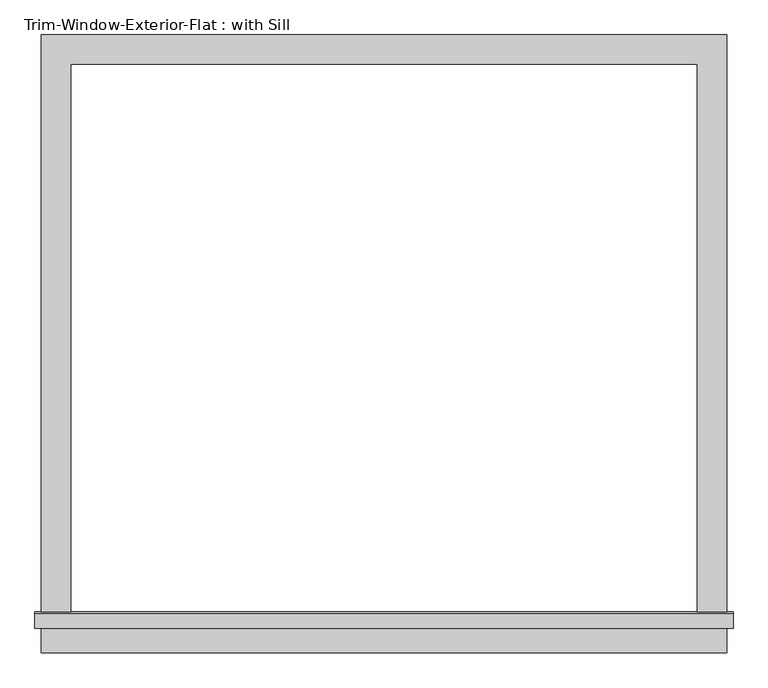
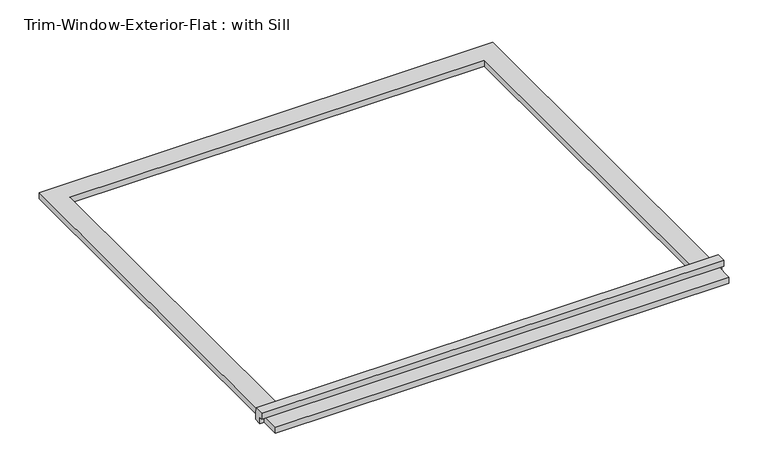
"""IFC4 building model written with IfcOpenShell, lengths in millimetres: proxy geometry, Trim-Window-Exterior-Flat : with Sill."""

from ifc_helpers import new_model, si_unit, frame, origin, origin_with_axes, place, context, project, spatial, polyline, outline, extrude, source, transform, mapped, element, save


def trim_window_exterior_flat_with_sill_f44f30ad(model_context):
    return source(origin(), model_context, "Body", "SweptSolid", [
        extrude(outline(polyline([(666.75, -1088.9823709), (666.75, -1146.1323709), (-666.75, -1146.1323709), (-666.75, -1088.9823709), (666.75, -1088.9823709)])), origin_with_axes(), (0.0, 0.0, 1.0), 19.05),
        extrude(outline(polyline([(-1098.55, 38.1), (-1069.2580645, 38.1), (-1066.8, 19.05), (-1066.8, 0.0), (-1088.9823709, 0.0), (-1088.9823709, 19.05), (-1098.55, 19.05), (-1098.55, 38.1)])), frame((-679.45, 0.0, 0.0), z_axis=(1.0, 0.0, 0.0), x_axis=(0.0, 1.0, 0.0)), (0.0, 0.0, 1.0), 1358.9),
        extrude(outline(polyline([(-666.75, 57.15), (666.75, 57.15), (666.75, -1066.8), (609.6, -1066.8), (609.6, 0.0), (-609.6, 0.0), (-609.6, -1066.8), (-666.75, -1066.8), (-666.75, 57.15)])), origin_with_axes(), (0.0, 0.0, 1.0), 19.05),
    ])


if __name__ == "__main__":
    model = new_model("IFC4")
    model_context = context("Model", 3, world=origin())
    ifc_project = project(units=[si_unit("LENGTHUNIT", "METRE", prefix="MILLI")], contexts=[model_context])
    site = spatial("IfcSite", under=ifc_project)
    building = spatial("IfcBuilding", under=site)
    placement = place(None, origin())
    trim_window_exterior_flat_with_sill_shape = trim_window_exterior_flat_with_sill_f44f30ad(model_context)
    element("IfcBuildingElementProxy", 1, Name="Trim-Window-Exterior-Flat : with Sill", ObjectType="Trim-Window-Exterior-Flat : with Sill", at=placement, inside=building, context=model_context, shape_type="MappedRepresentation", body=[
        mapped(trim_window_exterior_flat_with_sill_shape, transform((0.0, 0.0, 0.0), x_axis=(1.0, 0.0, 0.0), y_axis=(0.0, 1.0, 0.0), z_axis=(0.0, 0.0, 1.0))),
    ])
    save(model, "model.ifc")

# Revit data of these elements
# Type "Trim-Window-Exterior-Flat : with Sill"
#   Trim Width = 0' - 2 1/4"
#   Trim Thickness_Picture Frame = 0' - 1 1/4"
#   Trim Thickness_with Sill = 0' - 0 3/4"
#   Sill Thickness = 0' - 1 1/4"
#   Opening Width [instance default] = 2' - 0"
#   Opening Height [instance default] = 3' - 0"
#   Default Elevation = 4' - 0"
#   Sill = yes
#   Picture Frame = no
#   Trim Material [instance default] = none
# Element 1 (IfcBuildingElementProxy, "Trim-Window-Exterior-Flat : with Sill")
#   Opening Width = 4' - 0"
#   Opening Height = 3' - 6"
#   Trim Material = Clad - White
#   Materials on its faces: "Clad - White"
# Materials
#   "Clad - White": class "Wood", colour RGB 242 242 238, transparency 0, Cost = 0
